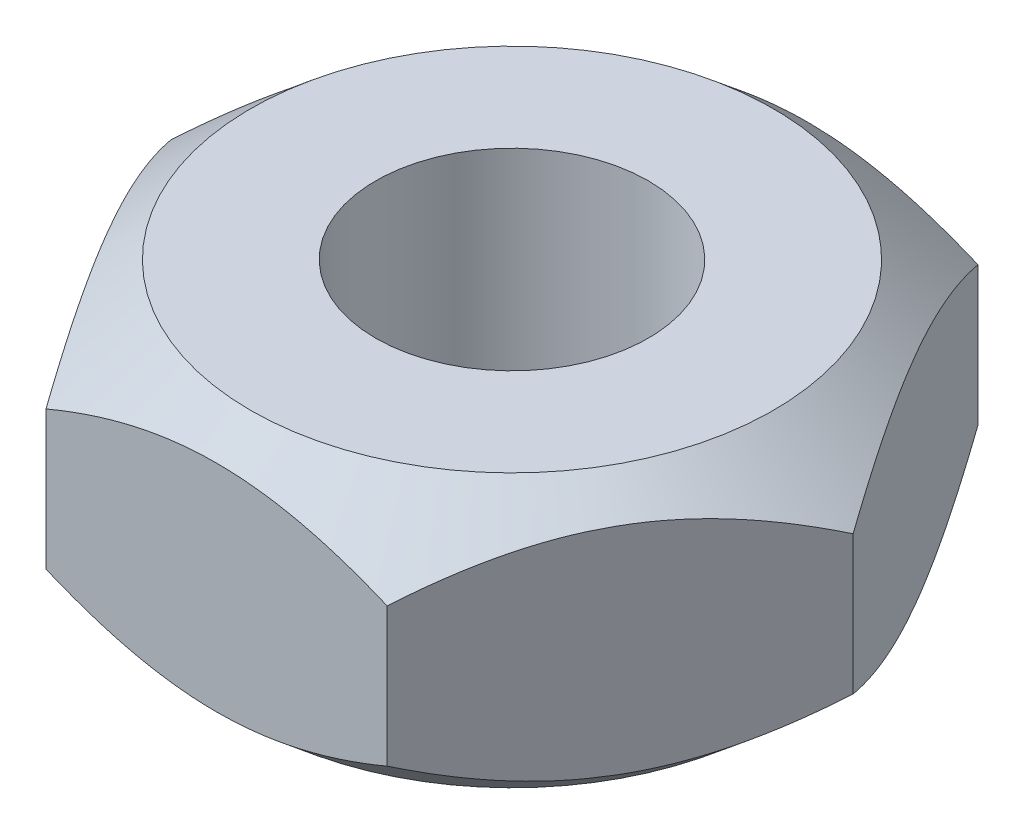
from build123d import *

# Parameters (mm, degrees)
HEX_NUT_PROFILE_R                     = 6
HEX_NUT_BODY_DEPTH                    = 6
CHAMFER_CIRCLE_23_OUTSIDE_W           = 98.006
CHAMFER_CIRCLE_23_OUTSIDE_H           = 93.984
CHAMFER_CIRCLE_23_OUTSIDE_R           = 11.5
CORNER_CHAMFER_50_DEPTH               = 24.202011407
CORNER_CHAMFER_50_DRAFT               = -50
CORNER_CHAMFER_MIRROR_COPY_1_SKETCH_W = 98.006
CORNER_CHAMFER_MIRROR_COPY_1_SKETCH_H = 93.984
CORNER_CHAMFER_MIRROR_COPY_1_SKETCH_R = 11.5
CORNER_CHAMFER_MIRROR_COPY_1_DEPTH    = 24.202011407
CORNER_CHAMFER_MIRROR_COPY_1_DRAFT    = -50


with BuildPart() as part:
    # Hex Nut Profile → Hex Nut Body (new, symmetric)
    with BuildSketch(Plane(origin=(0, 0, 0), x_dir=(1, 0, 0), z_dir=(0, 1, 0))):
        Polygon((15.011106999, 0), (7.505553499, 13), (-7.505553499, 13), (-15.011106999, 0), (-7.505553499, -13), (7.505553499, -13), align=None)
        with Locations(Location((0, 0, 0), (0, 0, 270))):
            Circle(HEX_NUT_PROFILE_R, mode=Mode.SUBTRACT)
    extrude(amount=HEX_NUT_BODY_DEPTH, both=True)


with BuildPart() as corner_chamfer_50_tool:
    # Chamfer Circle Ø23 outside → Corner Chamfer 50° (with draft: the straight prism first)
    with BuildSketch(Plane(origin=(0, 6, 0), x_dir=(1, 0, 0), z_dir=(0, 1, 0))):
        Rectangle(CHAMFER_CIRCLE_23_OUTSIDE_W, CHAMFER_CIRCLE_23_OUTSIDE_H)
        Circle(CHAMFER_CIRCLE_23_OUTSIDE_R, mode=Mode.SUBTRACT)
    extrude(amount=-CORNER_CHAMFER_50_DEPTH)
    # Corner Chamfer 50°: the draft: its side faces are tilted about the plane it starts from
    corner_chamfer_50_sides = [corner_chamfer_50_tool.faces().sort_by_distance(p)[0] for p in [
        (0, -6.101005704, 46.992),
        (49.003, -6.101005704, 0),
        (0, -6.101005704, -46.992),
        (-49.003, -6.101005704, 0),
        (-11.5, -6.101005704, 0),
    ]]
    draft(corner_chamfer_50_sides, Plane(origin=(0, 6, 0), x_dir=(1, 0, 0), z_dir=(0, 1, 0)), CORNER_CHAMFER_50_DRAFT)


with BuildPart() as part_1:
    add(part.part)

    # Corner Chamfer 50°: cut by corner_chamfer_50_tool
    add(corner_chamfer_50_tool.part, mode=Mode.SUBTRACT)


with BuildPart() as corner_chamfer_mirror_copy_1_tool:
    # Corner Chamfer Mirror copy 1 sketch → Corner Chamfer Mirror copy 1 (with draft: the straight prism first)
    with BuildSketch(Plane.XZ.offset(6)):
        Rectangle(CORNER_CHAMFER_MIRROR_COPY_1_SKETCH_W, CORNER_CHAMFER_MIRROR_COPY_1_SKETCH_H)
        Circle(CORNER_CHAMFER_MIRROR_COPY_1_SKETCH_R, mode=Mode.SUBTRACT)
    extrude(amount=-CORNER_CHAMFER_MIRROR_COPY_1_DEPTH)
    # Corner Chamfer Mirror copy 1: the draft: its side faces are tilted about the plane it starts from
    corner_chamfer_mirror_copy_1_sides = [corner_chamfer_mirror_copy_1_tool.faces().sort_by_distance(p)[0] for p in [
        (0, 6.101005704, 46.992),
        (49.003, 6.101005704, 0),
        (0, 6.101005704, -46.992),
        (-49.003, 6.101005704, 0),
        (-11.5, 6.101005704, 0),
    ]]
    draft(corner_chamfer_mirror_copy_1_sides, Plane.XZ.offset(6), CORNER_CHAMFER_MIRROR_COPY_1_DRAFT)


with BuildPart() as part_2:
    add(part_1.part)

    # Corner Chamfer Mirror copy 1: cut by corner_chamfer_mirror_copy_1_tool
    add(corner_chamfer_mirror_copy_1_tool.part, mode=Mode.SUBTRACT)


solid = part_2.part
